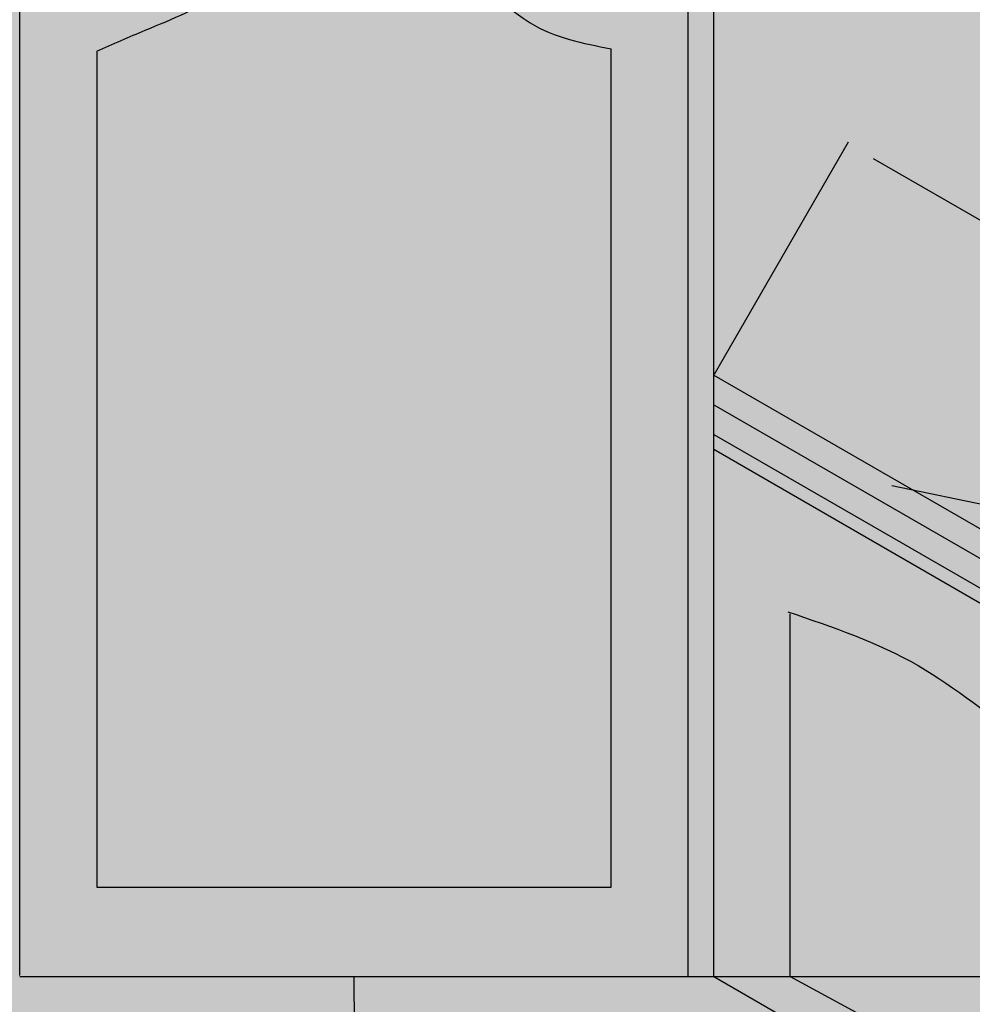
# Model space of a CAD drawing. Units: millimetres. Extents: x 78378 to 86415, y 148682 to 152721.
# Tile 14 of 18: x 80164 to 80806, y 151086 to 151749. Entities that reach past the tile are written whole.
import ezdxf

# ---------------------------------------------------------------- set-up
doc = ezdxf.new("R2010")
doc.units = ezdxf.units.MM
for name, color, linetype, lineweight in [('A-ANNO-DIMS', 2, 'Continuous', 18), ('A-FURN', 4, 'Continuous', 25), ('A-FURN-PATT', 32, 'Continuous', 13)]:
    doc.layers.add(name, color=color, linetype=linetype, lineweight=lineweight)
doc.styles.get("Standard").update_dxf_attribs({"font": 'arial.ttf'})
doc.dimstyles.new('ISO-25', dxfattribs={"dimtxt": 20, "dimasz": 20, "dimexe": 1.25, "dimexo": 0.625, "dimtad": 0, "dimdec": 1, "dimtxsty": 'Standard', "dimcen": 2.5, "dimadec": 0, "dimazin": 0, "dimtfac": 1, "dimtdec": 1, "dimtmove": 0, "dimatfit": 3, "dimfxl": 1, "dimarcsym": 0})

# ---------------------------------------------------------------- blocks, each defined once
blk = doc.blocks.new('*D2')
at = {"layer": 'A-ANNO-DIMS', "color": 0, "lineweight": -2, "transparency": 16777216}
for p, q in [((80389.2, 152255.55), (80340.72, 152339.52)), ((80324.02, 152328.44), (79430.33, 151812.47)), ((78540.01, 151298.44), (79377.29, 151781.84)), ((78570.55, 151205.55), (78522.07, 151289.52))]:
    blk.add_line(p, q, dxfattribs=at)
at = {"layer": 'A-ANNO-DIMS', "color": 0, "transparency": 16777216}
for points in [[(80322.36, 152331.33), (80325.69, 152325.55), (80341.34, 152338.44)], [(78538.34, 151301.33), (78541.68, 151295.55), (78522.69, 151288.44)]]:
    blk.add_solid(points, dxfattribs=at)
at = {"layer": 'Defpoints', "color": 0, "transparency": 16777216}
for p in [(80341.34, 152338.44), (80389.51, 152255.01), (78570.86, 151205.01)]:
    blk.add_point(p, dxfattribs=at)
at = {"layer": 'A-ANNO-DIMS', "color": 0, "transparency": 16777216, "insert": (79403.81, 151797.15), "char_height": 20, "attachment_point": 5, "rotation": 30}
blk.add_mtext('2100', dxfattribs=at)
blk = doc.blocks.new('*D3')
at = {"layer": 'A-ANNO-DIMS', "color": 0, "lineweight": -2, "transparency": 16777216}
for p, q in [((80389.83, 152255.55), (80445.17, 152351.41)), ((80461.87, 152340.33), (81144.68, 151946.11)), ((81812.87, 151560.33), (81195.8, 151916.6)), ((81775.47, 151455.55), (81830.81, 151551.41))]:
    blk.add_line(p, q, dxfattribs=at)
at = {"layer": 'A-ANNO-DIMS', "color": 0, "transparency": 16777216}
for points in [[(80463.53, 152343.22), (80460.2, 152337.44), (80444.55, 152350.33)], [(81814.53, 151563.22), (81811.2, 151557.44), (81830.19, 151550.33)]]:
    blk.add_solid(points, dxfattribs=at)
at = {"layer": 'Defpoints', "color": 0, "transparency": 16777216}
for p in [(80389.51, 152255.01), (81830.19, 151550.33), (81775.15, 151455.01)]:
    blk.add_point(p, dxfattribs=at)
at = {"layer": 'A-ANNO-DIMS', "color": 0, "transparency": 16777216, "insert": (81170.24, 151931.35), "char_height": 20, "attachment_point": 5, "rotation": 330}
blk.add_mtext('1600', dxfattribs=at)
blk = doc.blocks.new('*D17')
at = {"layer": 'A-ANNO-DIMS', "color": 0, "lineweight": -2, "transparency": 16777216}
for p, q in [((80164.03, 151825.55), (80073.72, 151981.97)), ((80057.03, 151970.89), (79823.5, 151836.07)), ((79550.4, 151678.39), (79783.93, 151813.22)), ((79622.77, 151513.05), (79532.46, 151669.47))]:
    blk.add_line(p, q, dxfattribs=at)
at = {"layer": 'A-ANNO-DIMS', "color": 0, "transparency": 16777216}
for points in [[(80055.36, 151973.78), (80058.69, 151968.01), (80074.35, 151980.89)], [(79548.73, 151681.28), (79552.07, 151675.51), (79533.08, 151668.39)]]:
    blk.add_solid(points, dxfattribs=at)
at = {"layer": 'Defpoints', "color": 0, "transparency": 16777216}
for p in [(80074.35, 151980.89), (80164.35, 151825.01), (79623.08, 151512.51)]:
    blk.add_point(p, dxfattribs=at)
at = {"layer": 'A-ANNO-DIMS', "color": 0, "transparency": 16777216, "insert": (79803.71, 151824.64), "char_height": 20, "attachment_point": 5, "rotation": 30}
blk.add_mtext('625', dxfattribs=at)
blk = doc.blocks.new('*D30')
at = {"layer": 'A-ANNO-DIMS', "color": 0, "lineweight": -2, "transparency": 16777216}
for p, q in [((80615.3, 151825.01), (81956.4, 151825.01)), ((81955.15, 151805.01), (81955.15, 151487.61)), ((81955.15, 151125.01), (81955.15, 151442.4)), ((80615.3, 151105.01), (81956.4, 151105.01))]:
    blk.add_line(p, q, dxfattribs=at)
at = {"layer": 'A-ANNO-DIMS', "color": 0, "transparency": 16777216}
for points in [[(81951.82, 151805.01), (81958.49, 151805.01), (81955.15, 151825.01)], [(81951.82, 151125.01), (81958.49, 151125.01), (81955.15, 151105.01)]]:
    blk.add_solid(points, dxfattribs=at)
at = {"layer": 'Defpoints', "color": 0, "transparency": 16777216}
for p in [(80614.68, 151825.01), (81955.15, 151825.01), (80614.68, 151105.01)]:
    blk.add_point(p, dxfattribs=at)
at = {"layer": 'A-ANNO-DIMS', "color": 0, "transparency": 16777216, "insert": (81955.15, 151465.01), "char_height": 20, "attachment_point": 5, "rotation": 90}
blk.add_mtext('720', dxfattribs=at)
blk = doc.blocks.new('*D31')
at = {"layer": 'A-ANNO-DIMS', "color": 0, "lineweight": -2, "transparency": 16777216}
for p, q in [((80632.31, 151510.55), (80722.63, 151666.97)), ((80739.32, 151655.89), (81005.53, 151502.19)), ((81310.9, 151325.89), (81044.68, 151479.59)), ((81238.53, 151160.55), (81328.84, 151316.97))]:
    blk.add_line(p, q, dxfattribs=at)
at = {"layer": 'A-ANNO-DIMS', "color": 0, "transparency": 16777216}
for points in [[(80740.99, 151658.78), (80737.65, 151653.01), (80722, 151665.89)], [(81312.56, 151328.78), (81309.23, 151323.01), (81328.22, 151315.89)]]:
    blk.add_solid(points, dxfattribs=at)
at = {"layer": 'Defpoints', "color": 0, "transparency": 16777216}
for p in [(80632, 151510.01), (81328.22, 151315.89), (81238.22, 151160.01)]:
    blk.add_point(p, dxfattribs=at)
at = {"layer": 'A-ANNO-DIMS', "color": 0, "transparency": 16777216, "insert": (81025.11, 151490.89), "char_height": 20, "attachment_point": 5, "rotation": 330}
blk.add_mtext('700', dxfattribs=at)
blk = doc.blocks.new('*D33')
at = {"layer": 'A-ANNO-DIMS', "color": 0, "lineweight": -2, "transparency": 16777216}
for p, q in [((80164.35, 151105.63), (80164.35, 152436.26)), ((80184.35, 152435.01), (80363.4, 152435.01)), ((80612, 152435.01), (80432.95, 152435.01)), ((80632, 151105.63), (80632, 152436.26))]:
    blk.add_line(p, q, dxfattribs=at)
at = {"layer": 'A-ANNO-DIMS', "color": 0, "transparency": 16777216}
for points in [[(80184.35, 152438.34), (80184.35, 152431.67), (80164.35, 152435.01)], [(80612, 152438.34), (80612, 152431.67), (80632, 152435.01)]]:
    blk.add_solid(points, dxfattribs=at)
at = {"layer": 'Defpoints', "color": 0, "transparency": 16777216}
for p in [(80632, 152435.01), (80164.35, 151105.01), (80632, 151105.01)]:
    blk.add_point(p, dxfattribs=at)
at = {"layer": 'A-ANNO-DIMS', "color": 0, "transparency": 16777216, "insert": (80398.17, 152435.01), "char_height": 20, "attachment_point": 5}
blk.add_mtext('467.7', dxfattribs=at)
blk = doc.blocks.new('*D69')
at = {"layer": 'A-ANNO-DIMS', "color": 0, "lineweight": -2, "transparency": 16777216}
for p, q in [((80751.91, 151435.61), (81200.94, 151342.55)), ((81427.33, 151295.63), (81220.52, 151338.49))]:
    blk.add_line(p, q, dxfattribs=at)
at = {"layer": 'A-ANNO-DIMS', "color": 0, "transparency": 16777216}
blk.add_solid([(81221.2, 151341.75), (81219.84, 151335.23), (81200.94, 151342.55)], dxfattribs=at)
at = {"layer": 'Defpoints', "color": 0, "transparency": 16777216}
for p in [(80751.91, 151435.61), (81200.94, 151342.55)]:
    blk.add_point(p, dxfattribs=at)
at = {"layer": 'A-ANNO-DIMS', "color": 0, "transparency": 16777216, "insert": (81470.35, 151286.71), "char_height": 20, "attachment_point": 5, "rotation": 348.29061}
blk.add_mtext('R458.6', dxfattribs=at)

msp = doc.modelspace()

# ---------------------------------------------------------------- hatches: boundary and pattern name
at = {"layer": 'A-FURN-PATT'}
h = msp.add_hatch(color=256, dxfattribs=at)
h.dxf.hatch_style = 1
h.paths.add_polyline_path([(78839.3276, 151040.0076), (78579.52, 151190.0076), (78579.52, 150470.0076), (78839.3276, 150320.0076)])
h.paths.add_polyline_path([(79073.1545, 150899.6469, 0.27777969), (79002.2645, 150996.3205, 0.79108393), (78917.9567, 150978.8719, 0.18044832), (78856.6481, 150853.0138), (78856.6481, 150350.6973), (79073.1545, 150484.318)])
h.paths.add_polyline_path([(79073.1545, 151175.0076), (78856.6481, 151050.0076), (78856.6481, 150853.0138, -0.18044832), (78917.9567, 150978.8719, -0.79108393), (79002.2645, 150996.3205, -0.27777969), (79073.1545, 150899.6469)])
h.paths.add_polyline_path([(79341.6224, 151350.0076), (79099.1352, 151490.0076), (78596.8405, 151200.0076), (78839.3276, 151060.0076)])
h.paths.add_polyline_path([(79904.5389, 151675.0076), (79662.0518, 151815.0076), (79099.1352, 151490.0076), (79341.6224, 151350.0076)])
h.paths.add_polyline_path([(80389.5131, 151955.0076), (80389.5131, 152235.0076), (79662.0518, 151815.0076), (79904.5389, 151675.0076)])
h.paths.add_polyline_path([(80389.5131, 151955.0076), (80164.3465, 151825.0076), (80164.3465, 151105.0076), (80614.6797, 151105.0076), (80614.6797, 151825.0076)])
edge = h.paths.add_edge_path(flags=16)
edge.add_spline(control_points=[(80216.308, 151728.251), (80227.1854, 151732.981), (80256.3301, 151745.6544), (80298.41, 151761.9595), (80340.2597, 151805.855), (80391.0771, 151782.0404), (80454.0396, 151805.7581), (80496.5007, 151742.4095), (80543.8218, 151733.4043), (80562.7182, 151729.8083)], knot_values=[0, 0, 0, 0, 35.54374676, 95.23575347, 136.36767513, 200.93298197, 236.72641081, 322.88993498, 380.17027367, 380.17027367, 380.17027367, 380.17027367], degree=3, periodic=0)
edge.add_line((80562.7182, 151729.8083), (80562.7182, 151165.0076))
edge.add_line((80562.7182, 151165.0076), (80216.308, 151165.0076))
edge.add_line((80216.308, 151165.0076), (80216.308, 151728.251))
h.paths.add_polyline_path([(80632.0002, 152095.0076), (80389.5131, 152235.0076), (80389.5131, 151955.0076), (80614.6797, 151825.0076), (80632.0002, 151815.0076)])
h.paths.add_polyline_path([(80867.7794, 151958.8805), (80632.0002, 152095.0076), (80632.0002, 151815.0076), (80632.0002, 151510.0076), (80867.7794, 151373.8805)])
h.paths.add_polyline_path([(80147.026, 151495.8203, 0.18918979), (80063.5671, 151597.7244, 0.78826136), (79979.2691, 151580.5832, 0.16072613), (79904.5389, 151413.5769), (79904.5389, 150955.0076), (80147.026, 151095.0076)])
h.paths.add_polyline_path([(80147.026, 151815.0076), (79904.5389, 151675.0076), (79904.5389, 151413.5769, -0.16072613), (79979.2691, 151580.5832, -0.78826136), (80063.5671, 151597.7244, -0.18918979), (80147.026, 151495.8203)])
h.paths.add_polyline_path([(79887.2184, 151645.0076), (79640.4011, 151502.5076), (79640.4011, 151262.3325, -0.16072613), (79715.1313, 151429.3387, -0.78826136), (79799.4294, 151446.48, -0.21290578), (79887.2184, 151328.7247)])
h.paths.add_polyline_path([(79799.4294, 151446.48, 0.78826136), (79715.1313, 151429.3387, 0.16072613), (79640.4011, 151262.3325), (79640.4011, 150822.5076), (79887.2184, 150965.0076), (79887.2184, 151328.7247, 0.21290578)])
h.paths.add_polyline_path([(79605.7601, 151482.5076), (79358.9429, 151340.0076), (79358.9429, 151100.0701, -0.16072613), (79433.6731, 151267.0764, -0.78826136), (79517.9711, 151284.2176, -0.21290578), (79605.7601, 151166.4623)])
h.paths.add_polyline_path([(79605.7601, 151166.4623, 0.21290578), (79517.9711, 151284.2176, 0.78826136), (79433.6731, 151267.0764, 0.16072613), (79358.9429, 151100.0701), (79358.9429, 150742.9831), (79419.0877, 150694.7323), (79605.7601, 150802.5076)])
edge = h.paths.add_edge_path(flags=0)
edge.add_spline(control_points=[(81152.4356, 151098.7676), (81105.7208, 151145.9466), (81038.6136, 151213.7208), (80882.3866, 151214.1938), (80797.4434, 151311.2997), (80711.8686, 151340.3754), (80681.7691, 151350.6023)], knot_values=[0, 0, 0, 0, 188.233441, 270.4032752, 445.45179201, 540.42858829, 540.42858829, 540.42858829, 540.42858829], degree=3, periodic=0)
edge.add_line((80683.4538, 151350.0269), (80683.4538, 151104.8792))
edge.add_line((80683.4538, 151104.8792), (81152.4356, 150851.399))
edge.add_line((81152.4356, 150851.399), (81152.4356, 151098.7676))
edge = h.paths.add_edge_path(flags=0)
edge.add_spline(control_points=[(80912.9018, 151027.1103), (80892.3742, 151034.1027), (80860.1663, 151045.0739), (80835.5097, 151068.1214), (80826.5679, 151076.4797)], knot_values=[0, 0, 0, 0, 63.98405104, 100.39142428, 100.39142428, 100.39142428, 100.39142428], degree=3, periodic=0)
edge.add_arc((80830.0414, 151081.2992), 5.9407, 100.9277276, 234.2187381, ccw=False)
edge.add_spline(control_points=[(80828.9152, 151087.1322), (80837.857, 151078.7739), (80862.5136, 151055.7263), (80894.7215, 151044.7552), (80915.2491, 151037.7628)], knot_values=[0, 0, 0, 0, 36.40737324, 100.39142428, 100.39142428, 100.39142428, 100.39142428], degree=3, periodic=0)
edge.add_arc((80914.7882, 151032.2795), 5.5026, -107.9540399, 85.195579, ccw=False)
h.paths.add_polyline_path([(81238.218, 151110.0076), (80632.0002, 151460.0076), (80632.0002, 151105.0076), (81238.218, 150755.0076)])
edge = h.paths.add_edge_path(flags=16)
edge.add_line((81152.4356, 150851.399), (80683.4538, 151104.8792))
edge.add_line((80683.4538, 151104.8792), (80683.4538, 151350.0279))
edge.add_spline(control_points=[(80681.7691, 151350.6023), (80711.8686, 151340.3754), (80797.4434, 151311.2997), (80882.3866, 151214.1938), (81038.6136, 151213.7208), (81105.7208, 151145.9466), (81152.4356, 151098.7676)], knot_values=[0, 0, 0, 0, 94.97679628, 270.02531309, 352.19514729, 540.42858829, 540.42858829, 540.42858829, 540.42858829], degree=3, periodic=0)
edge.add_line((81152.4356, 151098.7676), (81152.4356, 150851.399))
edge = h.paths.add_edge_path(flags=0)
edge.add_spline(control_points=[(80912.9018, 151027.1103), (80892.3742, 151034.1027), (80860.1663, 151045.0739), (80835.5097, 151068.1214), (80826.5679, 151076.4797)], knot_values=[0, 0, 0, 0, 63.98405104, 100.39142428, 100.39142428, 100.39142428, 100.39142428], degree=3, periodic=0)
edge.add_arc((80830.0414, 151081.2992), 5.9407, 100.9277276, 234.2187381, ccw=False)
edge.add_spline(control_points=[(80828.9152, 151087.1322), (80837.857, 151078.7739), (80862.5136, 151055.7263), (80894.7215, 151044.7552), (80915.2491, 151037.7628)], knot_values=[0, 0, 0, 0, 36.40737324, 100.39142428, 100.39142428, 100.39142428, 100.39142428], degree=3, periodic=0)
edge.add_arc((80914.7882, 151032.2795), 5.5026, -107.7417882, 85.195579, ccw=False)
h.paths.add_polyline_path([(81498.0256, 151255.0076), (81238.218, 151110.0076), (81238.218, 150755.0076), (81498.0256, 150905.0076)])
edge = h.paths.add_edge_path(flags=16)
edge.add_spline(control_points=[(81152.4356, 151098.7676), (81105.7208, 151145.9466), (81038.6136, 151213.7208), (80882.3866, 151214.1938), (80797.4434, 151311.2997), (80711.8686, 151340.3754), (80681.7691, 151350.6023)], knot_values=[0, 0, 0, 0, 188.233441, 270.4032752, 445.45179201, 540.42858829, 540.42858829, 540.42858829, 540.42858829], degree=3, periodic=0)
edge.add_line((80683.4538, 151350.0279), (80683.4538, 151104.8792))
edge.add_line((80683.4538, 151104.8792), (81152.4356, 150851.399))
edge.add_line((81152.4356, 150851.399), (81152.4356, 151098.7676))
h.paths.add_polyline_path([(81453.9904, 151280.4314), (80867.7794, 151618.8805), (80867.7794, 151373.8805), (81238.218, 151160.0076)])
edge = h.paths.add_edge_path(flags=16)
edge.add_line((81189.2304, 151297.6373), (81114.4166, 151300.2154))
edge.add_arc((81412.0967, 151394.0167), 312.1092, 179.7569303, 197.4900342, ccw=False)
edge.add_ellipse((81154.0183, 151392.0436), major_axis=(-54.0264, 3.6301), ratio=0.22179693, start_angle=0, end_angle=0.3517985, ccw=False)
edge.add_ellipse((81154.0183, 151392.0436), major_axis=(-54.0264, 3.6301), ratio=0.22179693, start_angle=180, end_angle=360, ccw=False)
edge.add_spline(control_points=[(81196.1844, 151321.9476), (81224.9802, 151347.1455), (81266.8846, 151383.8144), (81222.0354, 151387.0304), (81208.0056, 151388.0364)], knot_values=[0, 0, 0, 0, 75.09175173, 109.27580439, 109.27580439, 109.27580439, 109.27580439], degree=3, periodic=0)
edge.add_arc((80751.9112, 151435.6145), 458.5693, 342.4891602, 345.646172, ccw=False)
edge = h.paths.add_edge_path(flags=0)
edge.add_spline(control_points=[(81196.6193, 151323.657), (81197.893, 151324.7717), (81199.1654, 151325.8858), (81209.0233, 151334.5343), (81217.3959, 151341.9835), (81228.0928, 151352.5012), (81231.3883, 151355.9524), (81236.9493, 151362.4395), (81239.214, 151365.4773), (81241.4987, 151369.416), (81242.064, 151370.5542), (81242.9187, 151372.6971), (81243.2076, 151373.7015), (81243.5012, 151375.5539), (81243.5065, 151376.4), (81243.2432, 151377.9407), (81242.9775, 151378.6373), (81242.1402, 151379.937), (81241.5659, 151380.5416), (81240.2039, 151381.533), (81239.4963, 151381.9384), (81237.0619, 151383.0663), (81235.0242, 151383.6999), (81230.352, 151384.7569), (81227.7173, 151385.1826), (81221.9118, 151385.9145), (81218.7193, 151386.2133), (81213.7912, 151386.6115), (81212.1252, 151386.7359), (81209.6196, 151386.9181), (81208.7865, 151386.9779), (81207.9009, 151387.0432)], knot_values=[0.01548744, 0.01548744, 0.01548744, 0.01548744, 3.33787957, 3.33787957, 25.85130624, 25.85130624, 37.52811308, 37.52811308, 49.20491992, 49.20491992, 54.2850938, 54.2850938, 59.36526768, 59.36526768, 64.44544157, 64.44544157, 69.52561545, 69.52561545, 74.60578933, 74.60578933, 78.49366785, 78.49366785, 86.25567095, 86.25567095, 94.01767406, 94.01767406, 102.20226556, 102.20226556, 106.29456131, 106.29456131, 108.32522175, 108.32522175, 108.32522175, 108.32522175], degree=3, periodic=0)
edge = h.paths.add_edge_path(flags=16)
edge.add_arc((81034.1732, 151350.4693), 42.5822, 231.2679035, 306.151846, ccw=False)
edge.add_line((81007.5303, 151317.2517), (81007.5303, 151395.181))
edge.add_ellipse((81033.412, 151394.7791), major_axis=(-25.8816, 0.4538), ratio=0.23894509, start_angle=0, end_angle=0.1147075, ccw=False)
edge.add_ellipse((81033.412, 151394.7791), major_axis=(-25.8816, 0.4538), ratio=0.23894509, start_angle=181.1677709, end_angle=358.9476457, ccw=False)
edge.add_ellipse((81033.412, 151395.7791), major_axis=(-25.8816, 0.4538), ratio=0.23894509, start_angle=180, end_angle=360.1147075, ccw=False)
edge.add_ellipse((81033.412, 151395.7791), major_axis=(-25.8816, 0.4538), ratio=0.23894509, start_angle=178.9476457, end_angle=180, ccw=False)
edge.add_line((81059.2936, 151395.1778), (81059.2936, 151394.3772))
edge.add_ellipse((81033.412, 151394.7791), major_axis=(-25.8816, 0.4538), ratio=0.23894509, start_angle=180, end_angle=180.1147075, ccw=False)
edge.add_ellipse((81033.412, 151394.7791), major_axis=(-25.8816, 0.4538), ratio=0.23894509, start_angle=3.6903098, end_angle=176.4406503, ccw=False)
edge.add_line((81059.2936, 151393.3388), (81059.2936, 151316.086))
h.paths.add_polyline_path([(80951.9355, 151343.9568), (80909.6838, 151362.4635), (80904.0219, 151443.9615, -0.38133308), (80987.2169, 151411.3717)], flags=16)
h = msp.add_hatch(color=256, dxfattribs=at)
h.dxf.hatch_style = 1
h.paths.add_polyline_path([(80389.8136, 150935.1811), (80389.5131, 151105.0076), (80164.3465, 151105.0076), (79904.5389, 150955.0076), (79433.5848, 150683.1022), (79459.4128, 150662.3818), (79243.9048, 150537.9582), (79160.4069, 150518.1674), (78839.3276, 150320.0076), (78579.52, 150470.0076), (78570.8597, 150475.0076), (78570.8597, 150465.0076), (78570.8597, 149885.0076)])
h.paths.add_polyline_path([(80086.4042, 150460.0076), (79826.5966, 150610.0076), (78570.8597, 149885.0076), (78830.6674, 149735.0076)])
h.paths.add_polyline_path([(79540.8001, 150161.0557), (79217.3967, 149974.3386), (78980.9166, 150110.8705), (79304.32, 150297.5875)], flags=16)
h.paths.add_polyline_path([(79506.159, 150161.0557), (79217.3967, 149994.3386), (79015.5576, 150110.8705), (79304.32, 150277.5875)], flags=0)
edge = h.paths.add_edge_path(flags=0)
edge.add_arc((79247.8636, 150177.1541), 137.9799, 256.0025928, 293.5594109)
edge.add_arc((79240.7671, 150078.2605), 68.0855, 336.099104, 387.3696877)
edge.add_ellipse((79258.3074, 150109.4852), major_axis=(-42.6234, -1.6591), ratio=0.16042843, start_angle=0, end_angle=179.0977279, ccw=False)
edge.add_arc((79285.2112, 150074.2509), 77.2096, 155.1233104, 203.6557939)
edge = h.paths.add_edge_path(flags=0)
edge.add_ellipse((79258.6958, 150110.8297), major_axis=(-42.6234, -1.6591), ratio=0.16042843, start_angle=350.6039412, end_angle=356.2289762)
edge.add_line((79219.169, 150111.8937), (79218.3268, 150109.4141))
edge.add_arc((79262.4675, 150032.9602), 88.2813, 112.3931229, 120, ccw=False)
h.paths.add_polyline_path([(79287.0625, 150086.9703, -0.24770206), (79288.1967, 150077.2955, -0.39047651), (79265.4731, 150072.5438, -0.48726153), (79264.079, 150082.3769, 0.39560433)], flags=0)
h.paths.add_polyline_path([(80389.5131, 150935.0076), (79826.5966, 150610.0076), (80086.4042, 150460.0076), (80692.622, 150460.0076), (80952.4296, 150610.0076)])
edge = h.paths.add_edge_path(flags=16)
edge.add_ellipse((80392.4466, 150825.601), major_axis=(-133.0757, 7.722), ratio=0.42449957, start_angle=0, end_angle=360)
edge = h.paths.add_edge_path(flags=0)
edge.add_spline(control_points=[(80269.3541, 150832.7436), (80269.2919, 150831.672), (80269.3503, 150830.5922), (80269.7341, 150828.3361), (80270.0612, 150827.1587), (80271.0461, 150824.6748), (80271.7052, 150823.3692), (80273.4061, 150820.6503), (80274.4481, 150819.2381), (80276.9366, 150816.3509), (80278.3828, 150814.8762), (80282.5858, 150811.0913), (80285.6261, 150808.7701), (80292.6031, 150804.2267), (80296.5388, 150802.0041), (80305.195, 150797.7581), (80309.9151, 150795.7344), (80320.0112, 150791.96), (80325.387, 150790.2092), (80339.2162, 150786.315), (80347.9578, 150784.3563), (80366.0679, 150781.2568), (80375.4359, 150780.1158), (80394.3093, 150778.7158), (80403.8142, 150778.4568), (80422.4656, 150778.8319), (80431.6115, 150779.4662), (80449.0608, 150781.5838), (80457.3636, 150783.0675), (80472.6699, 150786.7766), (80479.6726, 150789.0033), (80490.1894, 150793.2813), (80494.1268, 150795.1967), (80501.0146, 150799.1885), (80503.9632, 150801.2651), (80508.2066, 150804.9015), (80509.73, 150806.4609), (80512.1996, 150809.4942), (80513.1456, 150810.9657), (80514.4291, 150813.5431), (80514.8436, 150814.6688), (80515.3984, 150816.8625), (80515.5405, 150817.9315), (80515.5801, 150820.098), (80515.4773, 150821.1978), (80514.9905, 150823.5062), (80514.6047, 150824.7154), (80513.4854, 150827.2641), (80512.7511, 150828.6027), (80510.8872, 150831.3809), (80509.7578, 150832.8196), (80507.0873, 150835.7513), (80505.5466, 150837.2439), (80501.0624, 150841.0944), (80497.8199, 150843.4576), (80490.4174, 150848.062), (80486.2582, 150850.3037), (80477.1448, 150854.5643), (80472.1909, 150856.5835), (80461.6275, 150860.3245), (80456.0182, 150862.0465), (80441.7332, 150865.8127), (80432.7885, 150867.6675), (80414.3391, 150870.5317), (80404.8349, 150871.5411), (80385.7707, 150872.6572), (80376.2113, 150872.764), (80357.5444, 150872.0728), (80348.4375, 150871.2748), (80331.1682, 150868.83), (80323.0064, 150867.1827), (80309.472, 150863.5363), (80303.8628, 150861.6593), (80293.8018, 150857.5401), (80289.3512, 150855.2969), (80282.7757, 150851.2345), (80280.3473, 150849.4579), (80276.2606, 150845.9127), (80274.604, 150844.1458), (80272.3157, 150841.1243), (80271.5358, 150839.8454), (80270.3496, 150837.3879), (80269.9417, 150836.2101), (80269.5065, 150834.2815), (80269.3988, 150833.5143), (80269.3541, 150832.7436)], knot_values=[0, 0, 0, 0, 0.09750046, 0.09750046, 0.19500092, 0.19500092, 0.29250138, 0.29250138, 0.39000184, 0.39000184, 0.4875023, 0.4875023, 0.63880322, 0.63880322, 0.79010415, 0.79010415, 0.94140507, 0.94140507, 1.092706, 1.092706, 1.3128171, 1.3128171, 1.5329282, 1.5329282, 1.7530393, 1.7530393, 1.97315041, 1.97315041, 2.19326151, 2.19326151, 2.41337261, 2.41337261, 2.56986063, 2.56986063, 2.72634866, 2.72634866, 2.84418658, 2.84418658, 2.96202451, 2.96202451, 3.06023388, 3.06023388, 3.15844325, 3.15844325, 3.25665261, 3.25665261, 3.35486198, 3.35486198, 3.45307135, 3.45307135, 3.55128072, 3.55128072, 3.64949009, 3.64949009, 3.80392773, 3.80392773, 3.95836537, 3.95836537, 4.11280301, 4.11280301, 4.26724064, 4.26724064, 4.48920349, 4.48920349, 4.71116635, 4.71116635, 4.9331292, 4.9331292, 5.15509205, 5.15509205, 5.3770549, 5.3770549, 5.55785361, 5.55785361, 5.73865232, 5.73865232, 5.87239556, 5.87239556, 6.00613879, 6.00613879, 6.109605, 6.109605, 6.2130712, 6.2130712, 6.28318531, 6.28318531, 6.28318531, 6.28318531], degree=3, periodic=0)
edge = h.paths.add_edge_path(flags=0)
edge.add_ellipse((80392.4466, 150825.601), major_axis=(-101.8398, 3.3923), ratio=0.40349248, start_angle=0, end_angle=360)
edge = h.paths.add_edge_path(flags=0)
edge.add_ellipse((80391.1657, 150858.3746), major_axis=(9.0882, -0.6733), ratio=0.35135413, start_angle=0, end_angle=360)
h.paths.add_polyline_path([(80952.4296, 150610.0076), (80692.622, 150460.0076), (81361.2342, 150073.9842), (81649.9628, 150052.7286), (81766.4935, 150120.0076), (81766.4935, 150140.0076), (81564.9025, 150256.3963), (81564.8884, 150096.1963), (81538.9076, 150111.1963), (81538.9217, 150271.3963)])
h.paths.add_polyline_path([(81539.0357, 151571.3305), (80867.7794, 151958.8805), (80867.7794, 151618.8805), (81498.0256, 151255.0076), (81498.0256, 150905.0076), (81238.218, 150755.0076), (81538.9488, 150581.3806)])
h.paths.add_polyline_path([(81766.4935, 151440.0076), (81565.0164, 151556.3305), (81564.9296, 150566.3806), (81766.4935, 150450.0076)])
edge = h.paths.add_edge_path()
edge.add_line((81564.9296, 150566.3806), (81564.9137, 150384.6289))
edge.add_ellipse((81552.1304, 150358.5718), major_axis=(52.6272, 3.506), ratio=0.49589905, start_angle=367.5169757, end_angle=420.0564686, ccw=False)
edge.add_ellipse((81552.1304, 150358.5718), major_axis=(52.6272, 3.506), ratio=0.49589905, start_angle=351.729742, end_angle=367.5169757, ccw=False)
edge.add_ellipse((81552.1304, 150345.5016), major_axis=(52.6272, 3.506), ratio=0.49589905, start_angle=352.5116949, end_angle=366.3006092, ccw=False)
edge.add_line((81603.4463, 150342.2039), (81603.5064, 150340.4475))
edge.add_ellipse((81552.1304, 150332.128), major_axis=(52.6272, 3.506), ratio=0.49589905, start_angle=353.6729654, end_angle=365.3867997, ccw=False)
edge.add_ellipse((81552.1304, 150332.128), major_axis=(52.6272, 3.506), ratio=0.49589905, start_angle=350.9388331, end_angle=353.6729654)
edge.add_line((81603.8688, 150329.855), (81604.0442, 150324.7302))
edge.add_ellipse((81552.1304, 150317.7418), major_axis=(52.6272, 3.506), ratio=0.49589905, start_angle=355.2176746, end_angle=363.8553364, ccw=False)
edge.add_ellipse((81552.1304, 150317.7418), major_axis=(52.6272, 3.506), ratio=0.49589905, start_angle=341.3250873, end_angle=355.2176746, ccw=False)
edge.add_ellipse((81552.1304, 150317.7418), major_axis=(52.6272, 3.506), ratio=0.49589905, start_angle=293.4661701, end_angle=341.3250873, ccw=False)
edge.add_line((81564.9057, 150292.9664), (81564.9025, 150256.3963))
edge.add_line((81564.9025, 150256.3963), (81766.4935, 150140.0076))
edge.add_line((81766.4935, 150140.0076), (81766.4935, 150450.0076))
edge.add_line((81766.4935, 150450.0076), (81564.9296, 150566.3806))
h.paths.add_polyline_path([(81525.5713, 150321.598), (81526.5985, 150321.3069), (81528.6771, 150320.947)])
h.paths.add_polyline_path([(81512.7903, 150326.1129), (81514.5058, 150325.3887), (81512.538, 150326.2678)])
h.paths.add_polyline_path([(81533.2148, 150320.1615), (81534.6952, 150319.9052), (81536.5995, 150319.7557)])
h.paths.add_polyline_path([(81518.622, 150323.6513), (81519.227, 150323.3959), (81521.289, 150322.8116)])
h.paths.add_polyline_path([(81501.2183, 150336.2599), (81500.3543, 150338.1339), (81499.7815, 150340.0494), (81499.5032, 150341.9955), (81499.5032, 150343.7257), (81499.7584, 150345.5905), (81500.2766, 150347.4549), (81501.0551, 150349.3095), (81501.0967, 150349.3937), (81501.1389, 150349.4778), (81500.9978, 150349.7496), (81500.8628, 150350.0225), (81499.5032, 150355.0658), (81499.9591, 150359.5002), (81501.8982, 150363.9083), (81505.2653, 150368.1646), (81509.9647, 150372.1482), (81515.8627, 150375.7459), (81522.7918, 150378.8553), (81530.555, 150381.3882), (81538.9315, 150383.2724), (81538.9488, 150581.3806), (80632.0002, 151105.0076), (80389.5131, 151105.0076), (80389.8142, 150934.8338), (80952.4296, 150610.0076), (81538.9217, 150271.3963), (81538.9234, 150291.7194), (81538.8752, 150291.721), (81530.1915, 150292.8239), (81522.1802, 150294.6904), (81515.0866, 150297.2633), (81509.8635, 150299.9959), (81505.6084, 150303.1351), (81502.419, 150306.6088), (81500.3683, 150310.3375), (81499.5032, 150314.2358), (81499.5032, 150315.9659), (81499.8206, 150318.1159), (81500.487, 150320.2634), (81501.4979, 150322.3941), (81500.487, 150324.4233), (81499.8206, 150326.5039), (81499.5032, 150328.622), (81499.5032, 150330.3521), (81499.7815, 150332.3262), (81500.3543, 150334.2992)])
h = msp.add_hatch(color=256, dxfattribs=at)
h.dxf.hatch_style = 1
h.paths.add_polyline_path([(79090.475, 151205.0076), (78839.3276, 151060.0076), (78839.3276, 150320.0076), (79090.475, 150475.0076)])
h.paths.add_polyline_path([(79073.1545, 151175.0076), (79073.1545, 150899.6469, -0.04544363), (79073.1545, 150878.5653), (79073.1545, 150484.318), (78856.6481, 150350.6973), (78856.6481, 150814.5249, -0.04815716), (78856.6481, 150853.0138), (78856.6481, 151050.0076)], flags=16)
h.paths.add_polyline_path([(79358.9429, 151340.0076), (79605.7601, 151482.5076), (79605.7601, 150802.5076), (79419.0877, 150694.7323), (79433.5848, 150683.1022), (79623.0806, 150792.5076), (79623.0806, 151512.5076), (79341.6224, 151350.0076), (79341.6224, 150756.8784), (79358.9429, 150742.9831)])
h.paths.add_polyline_path([(79341.6224, 151350.0076), (79090.475, 151205.0076), (79090.475, 150475.0076), (79160.4069, 150518.1674), (79107.7955, 150505.6973), (79107.7955, 151195.0076), (79109.5275, 151196.0076), (79324.3018, 151320.0076), (79324.3018, 150770.7736), (79341.6224, 150756.8784)])
h.paths.add_polyline_path([(79887.2184, 151645.0076), (79887.2184, 151665.0076), (79623.0806, 151512.5076), (79623.0806, 150792.5076), (79887.2184, 150945.0076), (79887.2184, 150965.0076), (79640.4011, 150822.5076), (79640.4011, 151502.5076)])
h.paths.add_polyline_path([(79904.5389, 151655.0076), (79887.2184, 151645.0076), (79887.2184, 150965.0076), (79904.5389, 150975.0076)])
h.paths.add_polyline_path([(80164.3465, 151825.0076), (80147.026, 151815.0076), (80147.026, 151095.0076), (80164.3465, 151105.0076)])
h.paths.add_polyline_path([(80632.0002, 151510.0076), (80632.0002, 151490.0076), (81238.218, 151140.0076), (81471.6045, 151270.2619), (81453.9904, 151280.4314), (81238.218, 151160.0076)])
h.paths.add_polyline_path([(80632.0002, 151490.0076), (80632.0002, 151470.0076), (81238.218, 151120.0076), (81489.2186, 151260.0924), (81471.6045, 151270.2619), (81238.218, 151140.0076)])
h.paths.add_polyline_path([(80632.0002, 151460.0076), (80632.0002, 151105.0076), (81238.218, 150755.0076), (81238.218, 151110.0076)])
edge = h.paths.add_edge_path(flags=16)
edge.add_spline(control_points=[(80681.7691, 151350.6023), (80711.8686, 151340.3754), (80797.4434, 151311.2997), (80882.3866, 151214.1938), (81038.6136, 151213.7208), (81105.7208, 151145.9466), (81152.4356, 151098.7676)], knot_values=[0, 0, 0, 0, 94.97679628, 270.02531309, 352.19514729, 540.42858829, 540.42858829, 540.42858829, 540.42858829], degree=3, periodic=0)
edge.add_line((81152.4356, 151098.7676), (81152.4356, 150851.399))
edge.add_line((81152.4356, 150851.399), (80683.4538, 151104.8792))
edge.add_line((80683.4538, 151104.8792), (80683.4538, 151350.027))
edge = h.paths.add_edge_path(flags=0)
edge.add_spline(control_points=[(80828.9152, 151087.1322), (80837.857, 151078.7739), (80862.5136, 151055.7263), (80894.7215, 151044.7552), (80915.2491, 151037.7628)], knot_values=[0, 0, 0, 0, 36.40737324, 100.39142428, 100.39142428, 100.39142428, 100.39142428], degree=3, periodic=0)
edge.add_arc((80914.7882, 151032.2795), 5.5026, -107.9540399, 85.195579, ccw=False)
edge.add_spline(control_points=[(80912.9018, 151027.1103), (80892.3742, 151034.1027), (80860.1663, 151045.0739), (80835.5097, 151068.1214), (80826.5679, 151076.4797)], knot_values=[0, 0, 0, 0, 63.98405104, 100.39142428, 100.39142428, 100.39142428, 100.39142428], degree=3, periodic=0)
edge.add_arc((80830.0414, 151081.2992), 5.9407, 100.9277276, 234.2187381, ccw=False)
h.paths.add_polyline_path([(80632.0002, 151815.0076), (80614.6797, 151825.0076), (80614.6797, 151105.0076), (80632.0002, 151105.0076)])
h.paths.add_polyline_path([(81498.0256, 151255.0076), (81489.2186, 151260.0924), (81238.218, 151120.0076), (80632.0002, 151470.0076), (80632.0002, 151460.0076), (81238.218, 151110.0076)])
h.paths.add_polyline_path([(78596.8405, 151200.0076), (78579.52, 151190.0076), (78839.3276, 151040.0076), (78839.3276, 151060.0076)])
h.paths.add_polyline_path([(78596.8405, 151200.0076), (78579.52, 151210.0076), (78579.52, 151190.0076)])
h.paths.add_polyline_path([(78579.52, 151210.0076), (78570.8597, 151205.0076), (78570.8597, 150475.0076), (78579.52, 150470.0076)])
h = msp.add_hatch(color=256, dxfattribs=at)
h.dxf.hatch_style = 1
h.set_gradient(color1=(255, 255, 255), color2=(199, 200, 202))
edge = h.paths.add_edge_path()
edge.add_spline(control_points=[(80562.7182, 151729.8083), (80543.8218, 151733.4043), (80496.5007, 151742.4095), (80454.0396, 151805.7581), (80391.0771, 151782.0404), (80340.2597, 151805.855), (80298.41, 151761.9595), (80256.3301, 151745.6544), (80227.1854, 151732.981), (80216.308, 151728.251)], knot_values=[0, 0, 0, 0, 57.28033869, 143.44386286, 179.2372917, 243.80259854, 284.9345202, 344.62652691, 380.17027367, 380.17027367, 380.17027367, 380.17027367], degree=3, periodic=0)
edge.add_line((80216.308, 151728.251), (80216.308, 151165.0076))
edge.add_line((80216.308, 151165.0076), (80562.7182, 151165.0076))
edge.add_line((80562.7182, 151165.0076), (80562.7182, 151729.8083))

# ---------------------------------------------------------------- linework, layer by layer
at = {"layer": 'A-FURN'}
for p, q in [((80632.0002, 151105.0076), (80632.0002, 152095.0076)), ((80614.6797, 151105.0076), (80614.6797, 151825.0076)), ((80216.308, 151728.251), (80216.308, 151165.0076)), ((80562.7182, 151165.0076), (80562.7182, 151729.8083)), ((80632.0002, 151510.0076), (81238.218, 151160.0076)), ((80632.0002, 151490.0076), (81238.218, 151140.0076)), ((80632.0002, 151470.0076), (81238.218, 151120.0076)), ((80632.0002, 151460.0076), (81238.218, 151110.0076)), ((80683.4538, 151104.8792), (80683.4538, 151349.2773)), ((80216.308, 151165.0076), (80562.7182, 151165.0076)), ((80164.3465, 151105.0076), (80632.0002, 151105.0076)), ((80389.5131, 151105.0076), (80389.907, 150882.375)), ((80632.0002, 151105.0076), (81538.9488, 150581.3806)), ((80683.4538, 151104.8792), (81152.4356, 150851.399))]:
    msp.add_line(p, q, dxfattribs=at)
for points, knots in [([(80216.308, 151728.251), (80227.1854, 151732.981), (80256.3301, 151745.6544), (80298.41, 151761.9595), (80340.2597, 151805.855), (80391.0771, 151782.0404), (80454.0396, 151805.7581), (80496.5007, 151742.4095), (80543.8218, 151733.4043), (80562.7182, 151729.8083)], [0, 0, 0, 0, 35.54374676, 95.23575347, 136.36767513, 200.93298197, 236.72641081, 322.88993498, 380.17027367, 380.17027367, 380.17027367, 380.17027367]), ([(80681.7691, 151350.6023), (80711.8686, 151340.3754), (80797.4434, 151311.2997), (80882.3866, 151214.1938), (81038.6136, 151213.7208), (81105.7208, 151145.9466), (81152.4356, 151098.7676)], [0, 0, 0, 0, 94.97679628, 270.02531309, 352.19514729, 540.42858829, 540.42858829, 540.42858829, 540.42858829])]:
    msp.add_open_spline(points, degree=3, knots=knots, dxfattribs=at)

# ---------------------------------------------------------------- dimensions: what is measured, and where the dimension line sits
at = {"layer": 'A-ANNO-DIMS'}
dim = msp.add_linear_dim(base=(80632.0002, 152435.0076), p1=(80164.3465, 151105.0076), p2=(80632.0002, 151105.0076), dimstyle='ISO-25', override={"dimdec": 1, "dimlfac": 1, "dimrnd": 0, "dimzin": 0, "dimdsep": 46, "dimlunit": 2}, dxfattribs=at)
dim.commit()
dim.dimension.update_dxf_attribs({"geometry": '*D33', "text_midpoint": (80398.1733, 152435.0076)})
for base, p1, p2, angle, picture, middle in [((81830.1884, 151550.3305), (80389.5131, 152255.0076), (81775.1537, 151455.0076), 330, '*D3', (81170.2376, 151931.3533)), ((80341.3443, 152338.4385), (78570.8597, 151205.0076), (80389.5131, 152255.0076), 30, '*D2', (79403.8116, 151797.1537))]:
    dim = msp.add_linear_dim(base=base, p1=p1, p2=p2, angle=angle, dimstyle='ISO-25', override={"dimclrd": 0, "dimclre": 0, "dimclrt": 0}, dxfattribs=at)
    dim.commit()
    dim.dimension.update_dxf_attribs({"geometry": picture, "text_midpoint": middle, "dimtype": 161})
for base, p1, p2, angle, picture, middle in [((80074.3465, 151980.8922), (79623.0806, 151512.5076), (80164.3465, 151825.0076), 30, '*D17', (79803.7135, 151824.6422)), ((81955.1537, 151825.0076), (80614.6797, 151105.0076), (80614.6797, 151825.0076), 90, '*D30', (81955.1537, 151465.0076)), ((81328.218, 151315.8922), (80632.0002, 151510.0076), (81238.218, 151160.0076), 330, '*D31', (81025.1091, 151490.8922))]:
    dim = msp.add_linear_dim(base=base, p1=p1, p2=p2, angle=angle, dimstyle='ISO-25', override={"dimdec": 0, "dimlfac": 1, "dimrnd": 0, "dimzin": 0, "dimdsep": 46, "dimlunit": 2}, dxfattribs=at)
    dim.commit()
    dim.dimension.update_dxf_attribs({"geometry": picture, "text_midpoint": middle})
dim = msp.add_radius_dim(center=(80751.9112, 151435.6145), mpoint=(81200.9374, 151342.5489), dimstyle='ISO-25', override={"dimdec": 1, "dimlfac": 1, "dimrnd": 0, "dimzin": 0, "dimdsep": 46, "dimlunit": 2}, dxfattribs=at)
dim.commit()
dim.dimension.update_dxf_attribs({"geometry": '*D69', "text_midpoint": (81470.3532, 151286.7096), "dimtype": 164})

doc.saveas('drawing.dxf')
